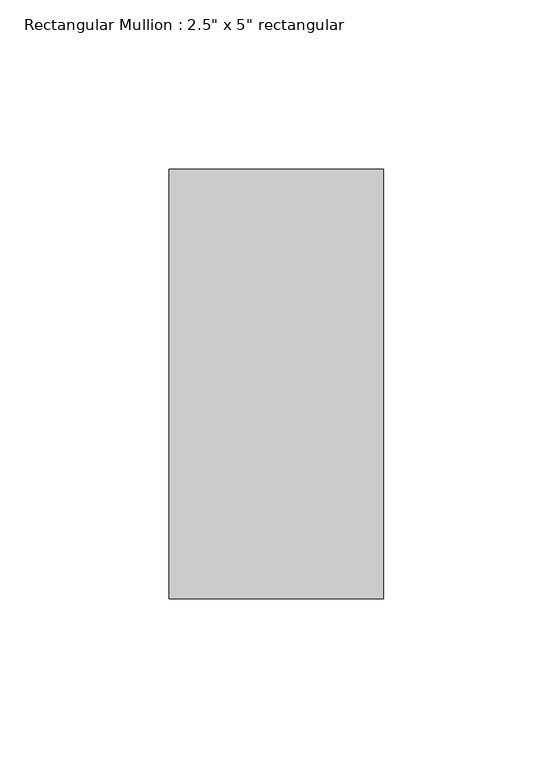
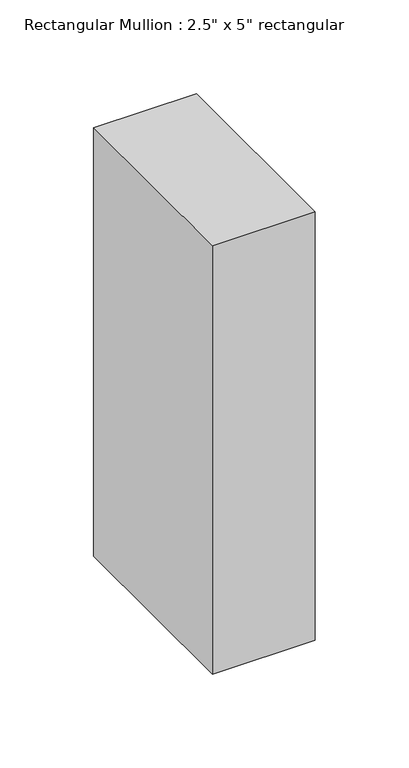
"""IFC4 building model written with IfcOpenShell, lengths in millimetres: member geometry."""

from ifc_helpers import new_model, si_unit, frame, origin, place, context, project, spatial, polyline, outline, extrude, source, transform, mapped, element, save


def member_d3323a85(model_context):
    return source(origin(), model_context, "Body", "SweptSolid", [
        extrude(outline(polyline([(0.0, 63.5), (0.0, -63.5), (-63.5, -63.5), (-63.5, 63.5), (0.0, 63.5)])), frame((0.0, 0.0, -279.4), z_axis=(0.0, 0.0, 1.0), x_axis=(1.0, 0.0, 0.0)), (0.0, 0.0, 1.0), 279.4),
    ])


if __name__ == "__main__":
    model = new_model("IFC4")
    model_context = context("Model", 3, world=origin())
    ifc_project = project(units=[si_unit("LENGTHUNIT", "METRE", prefix="MILLI")], contexts=[model_context])
    site = spatial("IfcSite", under=ifc_project)
    building = spatial("IfcBuilding", under=site)
    placement = place(None, origin())
    member_shape = member_d3323a85(model_context)
    element("IfcMember", 1, ObjectType="Rectangular Mullion : 2.5\" x 5\" rectangular", at=placement, inside=building, context=model_context, shape_type="MappedRepresentation", body=[
        mapped(member_shape, transform((0.0, 0.0, 0.0), x_axis=(1.0, 0.0, 0.0), y_axis=(0.0, 1.0, 0.0), z_axis=(0.0, 0.0, 1.0))),
    ])
    save(model, "model.ifc")

# Revit data of these elements
# Type "Rectangular Mullion : 2.5\" x 5\" rectangular"
#   built-in parameter 1007304 = 0.416667 (stored number, unit not read)
#   built-in parameter 1007301 = 0.104167 (stored number, unit not read)
#   built-in parameter 1007300 = 0.104167 (stored number, unit not read)
# Element 1 (IfcMember, "Rectangular Mullion : 2.5\" x 5\" rectangular")
#   Materials on its faces: "Aluminum"
# Materials
#   "Aluminum": class "Metal", colour RGB 247 247 247, transparency 0, Description = "Aluminum 6061", Cost = 0
